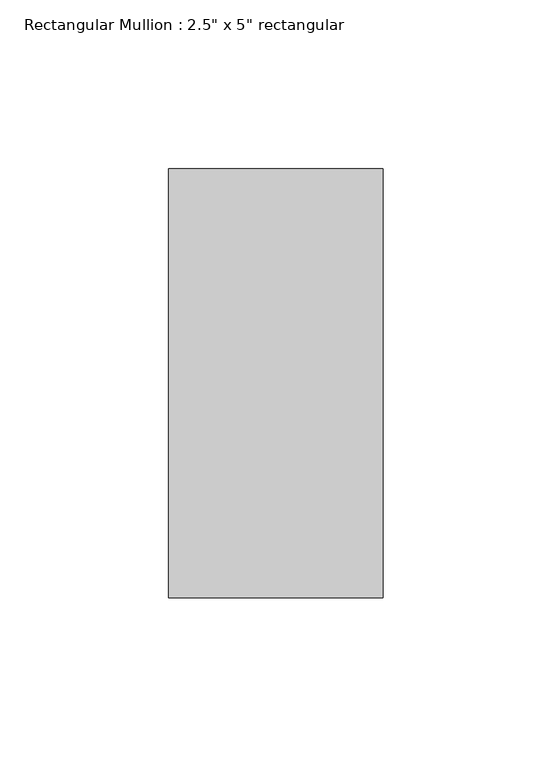
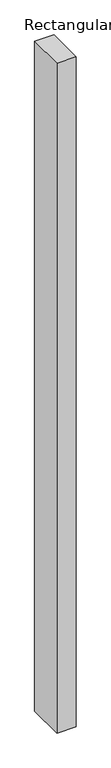
"""IFC4 building model written with IfcOpenShell, lengths in millimetres: member geometry."""

from ifc_helpers import new_model, si_unit, frame, origin, place, context, project, spatial, polyline, outline, extrude, source, transform, mapped, element, save


def member_9597caa3(model_context):
    return source(origin(), model_context, "Body", "SweptSolid", [
        extrude(outline(polyline([(31.75, 63.5), (31.75, -63.5), (-31.75, -63.5), (-31.75, 63.5), (31.75, 63.5)])), frame((0.0, 0.0, -2343.15), z_axis=(0.0, 0.0, 1.0), x_axis=(1.0, 0.0, 0.0)), (0.0, 0.0, 1.0), 2343.15),
    ])


if __name__ == "__main__":
    model = new_model("IFC4")
    model_context = context("Model", 3, world=origin())
    ifc_project = project(units=[si_unit("LENGTHUNIT", "METRE", prefix="MILLI")], contexts=[model_context])
    site = spatial("IfcSite", under=ifc_project)
    building = spatial("IfcBuilding", under=site)
    placement = place(None, origin())
    member_shape = member_9597caa3(model_context)
    element("IfcMember", 1, ObjectType="Rectangular Mullion : 2.5\" x 5\" rectangular", at=placement, inside=building, context=model_context, shape_type="MappedRepresentation", body=[
        mapped(member_shape, transform((0.0, 0.0, 0.0), x_axis=(1.0, 0.0, 0.0), y_axis=(0.0, 1.0, 0.0), z_axis=(0.0, 0.0, 1.0))),
    ])
    save(model, "model.ifc")

# Revit data of these elements
# Type "Rectangular Mullion : 2.5\" x 5\" rectangular"
#   built-in parameter 1007304 = 0.416667 (stored number, unit not read)
#   built-in parameter 1007301 = 0.104167 (stored number, unit not read)
#   built-in parameter 1007300 = 0.104167 (stored number, unit not read)
# Element 1 (IfcMember, "Rectangular Mullion : 2.5\" x 5\" rectangular")
#   Materials on its faces: "Aluminum"
# Materials
#   "Aluminum": class "Metal", colour RGB 247 247 247, transparency 0, Description = "Aluminum 6061", Cost = 0
